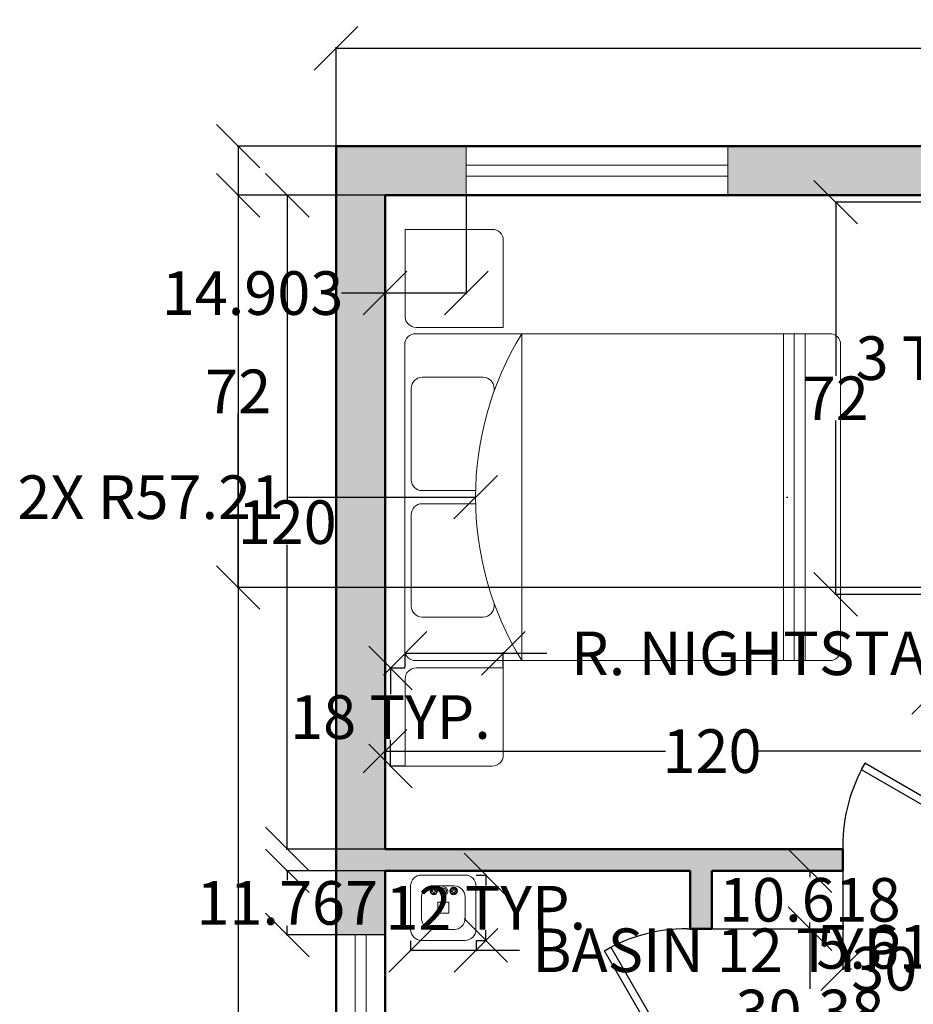
# Model space of a CAD drawing. Units: inches. Extents: x -87 to 308, y -349 to 42.
# Tile 2 of 6: x -45 to 119, y -139 to 42. Entities that reach past the tile are written whole.
import ezdxf

# ---------------------------------------------------------------- set-up
doc = ezdxf.new("R2010")
doc.units = ezdxf.units.IN
doc.header["$MEASUREMENT"] = 0
for name, color, linetype, lineweight in [('A-ANNO-DIMS', 2, 'Continuous', 18), ('A-DOOR', 3, 'Continuous', 25), ('A-FLOR-FIXT', 9, 'Continuous', 18), ('A-FURN', 8, 'Continuous', 18), ('A-GLAZ', 4, 'Continuous', 18), ('A-WALL', 7, 'Continuous', 50), ('A-WALL-PATT', 251, 'Continuous', 13)]:
    doc.layers.add(name, color=color, linetype=linetype, lineweight=lineweight)
doc.styles.get("Standard").update_dxf_attribs({"font": 'arial.ttf'})
doc.dimstyles.get("Standard").update_dxf_attribs({"dimtxt": 8, "dimasz": 8, "dimexe": 0.18, "dimexo": 0.0625, "dimgap": 0.09, "dimtad": 0, "dimtih": 1, "dimtoh": 1, "dimdec": 0, "dimzin": 0, "dimdsep": 46, "dimlunit": 4, "dimtxsty": 'Standard', "dimblk": 'OBLIQUE', "dimcen": 0.09, "dimadec": 0, "dimazin": 0, "dimtfac": 1, "dimtdec": 0, "dimtofl": 0, "dimtmove": 0, "dimatfit": 3, "dimldrblk": 'OBLIQUE', "dimfxl": 1, "dimtolj": 1, "dimtzin": 0, "dimarcsym": 0})

# ---------------------------------------------------------------- blocks, each defined once
blk = doc.blocks.new('*U6')
for p, q in [((-40, 0), (-40, 6)), ((0, 0), (0, 6))]:
    blk.add_line(p, q)
blk.add_lwpolyline([(0, 0), (-34.64, -20), (-35.52, -18.48), (-0.87, 1.52)], close=True)
blk.add_arc((0, 0), 40, 180, 210)
blk = doc.blocks.new('*U5')
for p, q in [((0, 0), (0, -6)), ((-40, 0), (-40, -6))]:
    blk.add_line(p, q)
blk.add_lwpolyline([(0, 0), (-34.64, 20), (-35.52, 18.48), (-0.88, -1.52)], close=True)
blk.add_arc((0, 0), 40, 150, 180)
blk = doc.blocks.new('Bed - Queen')
for p, q in [((2, 0), (58, 0)), ((10, -1.2), (26.8, -1.2)), ((33.2, -1.2), (50, -1.2)), ((0, -78), (0, -2)), ((8, -14.4), (8, -3.2)), ((28.8, -3.2), (28.8, -13.02)), ((31.2, -13.02), (31.2, -3.2)), ((52, -3.2), (52, -14.4)), ((60, -2), (60, -78)), ((10.58, -16.4), (10, -16.4)), ((50, -16.4), (49.42, -16.4)), ((60, -21.5), (0, -21.5)), ((0, -69.5), (60, -69.5)), ((0, -71.5), (60, -71.5)), ((0, -73.5), (60, -73.5)), ((58, -80), (2, -80))]:
    blk.add_line(p, q)
for centre, radius, start, end in [((58, -2), 2, 0, 90), ((2, -2), 2, 90, 180), ((10, -3.2), 2, 90, 180), ((26.8, -3.2), 2, 0, 90), ((33.2, -3.2), 2, 90, 180), ((50, -3.2), 2, 0, 90), ((30, -70.21), 57.21, 58.3725, 121.6275), ((10, -14.4), 2, 180, 270), ((50, -14.4), 2, 270, 0), ((2, -78), 2, 180, 270), ((58, -78), 2, 270, 0)]:
    blk.add_arc(centre, radius, start, end)
blk = doc.blocks.new('Faucet - Bathroom top')
for p, q in [((-4.107, 0.125), (-4.375, 0.125)), ((-3.75, 0.4788), (-3.75, 0.75)), ((-3.5, 0.482), (-3.5, 0.75)), ((-3.1461, 0.125), (-2.875, 0.125)), ((3.143, 0.125), (2.875, 0.125)), ((3.5, 0.4788), (3.5, 0.75)), ((3.75, 0.482), (3.75, 0.75)), ((4.1039, 0.125), (4.375, 0.125)), ((-4.1039, -0.125), (-4.375, -0.125)), ((-3.75, -0.4821), (-3.75, -0.75)), ((-3.5, -0.4789), (-3.5, -0.75)), ((-3.143, -0.125), (-2.875, -0.125)), ((-0.5, -0.8639), (-0.5, -4.5)), ((0.5, -4.5), (0.5, -0.8631)), ((3.1461, -0.125), (2.875, -0.125)), ((3.5, -0.4821), (3.5, -0.75)), ((3.75, -0.4789), (3.75, -0.75)), ((4.107, -0.125), (4.375, -0.125))]:
    blk.add_line(p, q)
for centre, radius in [((-3.625, 0), 1.375), ((-4.625, 0), 0.2795), ((-3.625, 0), 0.5), ((-3.625, 1), 0.2795), ((-2.625, 0), 0.2795), ((0, 0), 0.5), ((3.625, 0), 1.375), ((2.625, 0), 0.2795), ((3.625, 0), 0.5), ((3.625, 1), 0.2795), ((4.625, 0), 0.2795), ((-3.625, -1), 0.2795), ((3.625, -1), 0.2795)]:
    blk.add_circle(centre, radius)
for centre, radius, start, end in [((-3.625, 0), 1, 105.2407, 164.2093), ((-3.625, 0), 1, 16.44125, 74.07887), ((0, 0), 1.5, 289.6514, 250.3603), ((0, 0), 1, 300.3431, 239.7554), ((3.625, 0), 1, 106.12, 164.0884), ((3.625, 0), 1, 16.23422, 73.90469), ((-3.625, 0), 1, 196.2342, 253.9047), ((-3.625, 0), 1, 286.12, 344.0884), ((3.625, 0), 1, 196.4413, 254.0789), ((3.625, 0), 1, 285.2407, 344.2093), ((0, -4.5), 0.5, 180, 0)]:
    blk.add_arc(centre, radius, start, end)
blk = doc.blocks.new('WIN-48IN')
for p, q in [((0, 5.5), (48, 5.5)), ((0, 3.5), (48, 3.5))]:
    blk.add_line(p, q)
for points in [[(0, 0), (0, 9)], [(48, 9), (48, 0)]]:
    blk.add_lwpolyline(points)
blk = doc.blocks.new('WIN-24IN')
for p, q in [((0, 5.5), (24, 5.5)), ((0, 3.5), (24, 3.5))]:
    blk.add_line(p, q)
for points in [[(0, 0), (0, 9)], [(24, 9), (24, 0)]]:
    blk.add_lwpolyline(points)
blk = doc.blocks.new('LAVATORY-12IN')
for p, q in [((2, 12), (10, 12)), ((0, 2), (0, 10)), ((4, 10), (8, 10)), ((12, 10), (12, 2)), ((2, 4), (2, 8)), ((10, 8), (10, 4)), ((5, 7), (7, 7)), ((5, 5), (5, 7)), ((7, 7), (7, 5)), ((7, 5), (5, 5)), ((8, 2), (4, 2)), ((10, 0), (2, 0))]:
    blk.add_line(p, q)
for centre, start, end in [((2, 10), 90, 180), ((10, 10), 0, 90), ((4, 8), 90, 180), ((8, 8), 0, 90), ((4, 4), 180, 270), ((8, 4), 270, 0), ((2, 2), 180, 270), ((10, 2), 270, 0)]:
    blk.add_arc(centre, 2, start, end)
blk = doc.blocks.new('NIGHTSTAND-18IN-L')
blk.add_lwpolyline([(2, 0), (18, 0), (18, 16, 0.414214), (16, 18), (0, 18), (0, 2, 0.414214)], format="xyb", close=True)
blk = doc.blocks.new('NIGHTSTAND-18IN-R')
blk.add_lwpolyline([(0, 0), (16, 0, 0.414214), (18, 2), (18, 18), (2, 18, 0.414214), (0, 16)], format="xyb", close=True)
blk = doc.blocks.new('_Oblique')
at = {"color": 0, "linetype": 'ByBlock', "lineweight": -2}
blk.add_line((-0.5, -0.5), (0.5, 0.5), dxfattribs=at)
blk = doc.blocks.new('*D32')
at = {"layer": 'A-ANNO-DIMS', "color": 0, "lineweight": -2, "transparency": 16777216}
for p, q in [((147.96, -20.57), (139.96, -20.57)), ((147.96, -21.27), (147.96, -20.39)), ((151.23, -20.57), (147.96, -20.57)), ((151.23, -21.27), (151.23, -20.39))]:
    blk.add_line(p, q, dxfattribs=at)
at = {"layer": 'Defpoints', "color": 0, "transparency": 16777216}
for p in [(147.96, -20.57), (147.96, -21.33), (151.23, -21.33)]:
    blk.add_point(p, dxfattribs=at)
at = {"layer": 'A-ANNO-DIMS', "color": 0, "lineweight": -2, "transparency": 16777216, "xscale": 8, "yscale": 8, "zscale": 8, "rotation": 180}
blk.add_blockref('_Oblique', (147.96, -20.57), dxfattribs=at)
at = {"layer": 'A-ANNO-DIMS', "color": 0, "lineweight": -2, "transparency": 16777216, "xscale": 8, "yscale": 8, "zscale": 8}
blk.add_blockref('_Oblique', (151.23, -20.57), dxfattribs=at)
at = {"layer": 'A-ANNO-DIMS', "color": 0, "transparency": 16777216, "insert": (123.51, -20.57), "char_height": 8, "attachment_point": 5}
blk.add_mtext('\\A1;3 TYP.', dxfattribs=at)
blk = doc.blocks.new('*D33')
at = {"layer": 'A-ANNO-DIMS', "color": 0, "lineweight": -2, "transparency": 16777216}
for p, q in [((26.45, -127.5), (26.45, -129.42)), ((38.45, -127.5), (38.45, -129.42)), ((26.45, -129.24), (38.45, -129.24)), ((38.45, -129.24), (46.45, -129.24))]:
    blk.add_line(p, q, dxfattribs=at)
at = {"layer": 'Defpoints', "color": 0, "transparency": 16777216}
for p in [(26.45, -127.44), (38.45, -127.44), (38.45, -129.24)]:
    blk.add_point(p, dxfattribs=at)
at = {"layer": 'A-ANNO-DIMS', "color": 0, "lineweight": -2, "transparency": 16777216, "xscale": 8, "yscale": 8, "zscale": 8, "rotation": 180}
blk.add_blockref('_Oblique', (26.45, -129.24), dxfattribs=at)
at = {"layer": 'A-ANNO-DIMS', "color": 0, "lineweight": -2, "transparency": 16777216, "xscale": 8, "yscale": 8, "zscale": 8}
blk.add_blockref('_Oblique', (38.45, -129.24), dxfattribs=at)
at = {"layer": 'A-ANNO-DIMS', "color": 0, "transparency": 16777216, "insert": (84.15, -129.24), "char_height": 8, "attachment_point": 5}
blk.add_mtext('\\A1;BASIN 12 TYP.', dxfattribs=at)
blk = doc.blocks.new('*D34')
at = {"layer": 'A-ANNO-DIMS', "color": 0, "lineweight": -2, "transparency": 16777216}
for p, q in [((38.51, -115.44), (40.43, -115.44)), ((40.25, -115.44), (40.25, -117.33)), ((40.25, -127.44), (40.25, -125.54)), ((38.51, -127.44), (40.43, -127.44))]:
    blk.add_line(p, q, dxfattribs=at)
at = {"layer": 'Defpoints', "color": 0, "transparency": 16777216}
for p in [(38.45, -115.44), (40.25, -115.44), (38.45, -127.44)]:
    blk.add_point(p, dxfattribs=at)
at = {"layer": 'A-ANNO-DIMS', "color": 0, "lineweight": -2, "transparency": 16777216, "xscale": 8, "yscale": 8, "zscale": 8}
for p, rotation in [((40.25, -115.44), 90), ((40.25, -127.44), 270)]:
    blk.add_blockref('_Oblique', p, dxfattribs=dict(at, rotation=rotation))
at = {"layer": 'A-ANNO-DIMS', "color": 0, "transparency": 16777216, "insert": (40.25, -121.44), "char_height": 8, "attachment_point": 5}
blk.add_mtext('\\A1;12 TYP.', dxfattribs=at)
blk = doc.blocks.new('*D37')
at = {"layer": 'A-ANNO-DIMS', "color": 0, "lineweight": -2, "transparency": 16777216}
for p, q in [((25.45, -77.37), (25.45, -74.56)), ((25.45, -74.74), (43.45, -74.74)), ((43.45, -77.37), (43.45, -74.56)), ((43.45, -74.74), (51.45, -74.74))]:
    blk.add_line(p, q, dxfattribs=at)
at = {"layer": 'Defpoints', "color": 0, "transparency": 16777216}
for p in [(43.45, -74.74), (25.45, -77.44), (43.45, -77.44)]:
    blk.add_point(p, dxfattribs=at)
at = {"layer": 'A-ANNO-DIMS', "color": 0, "lineweight": -2, "transparency": 16777216, "xscale": 8, "yscale": 8, "zscale": 8, "rotation": 180}
blk.add_blockref('_Oblique', (25.45, -74.74), dxfattribs=at)
at = {"layer": 'A-ANNO-DIMS', "color": 0, "lineweight": -2, "transparency": 16777216, "xscale": 8, "yscale": 8, "zscale": 8}
blk.add_blockref('_Oblique', (43.45, -74.74), dxfattribs=at)
at = {"layer": 'A-ANNO-DIMS', "color": 0, "transparency": 16777216, "insert": (115.81, -74.74), "char_height": 8, "attachment_point": 5}
blk.add_mtext('\\A1;R. NIGHTSTAND 18 TYP.', dxfattribs=at)
blk = doc.blocks.new('*D38')
at = {"layer": 'A-ANNO-DIMS', "color": 0, "lineweight": -2, "transparency": 16777216}
for p, q in [((25.38, -77.44), (22.57, -77.44)), ((22.75, -77.44), (22.75, -82.26)), ((22.75, -95.44), (22.75, -90.61)), ((25.38, -95.44), (22.57, -95.44))]:
    blk.add_line(p, q, dxfattribs=at)
at = {"layer": 'Defpoints', "color": 0, "transparency": 16777216}
for p in [(22.75, -77.44), (25.45, -77.44), (25.45, -95.44)]:
    blk.add_point(p, dxfattribs=at)
at = {"layer": 'A-ANNO-DIMS', "color": 0, "lineweight": -2, "transparency": 16777216, "xscale": 8, "yscale": 8, "zscale": 8}
for p, rotation in [((22.75, -77.44), 90), ((22.75, -95.44), 270)]:
    blk.add_blockref('_Oblique', p, dxfattribs=dict(at, rotation=rotation))
at = {"layer": 'A-ANNO-DIMS', "color": 0, "transparency": 16777216, "insert": (22.75, -86.44), "char_height": 8, "attachment_point": 5}
blk.add_mtext('\\A1;18 TYP.', dxfattribs=at)
blk = doc.blocks.new('*D47')
at = {"layer": 'A-ANNO-DIMS', "color": 0, "lineweight": -2, "transparency": 16777216}
for p, q in [((12.76, 18.39), (12.76, 36.48)), ((12.76, 36.3), (120.78, 36.3)), ((246.76, 36.3), (138.74, 36.3)), ((246.76, 18.39), (246.76, 36.48))]:
    blk.add_line(p, q, dxfattribs=at)
at = {"layer": 'Defpoints', "color": 0, "transparency": 16777216}
for p in [(246.76, 36.3), (12.76, 18.33), (246.76, 18.33)]:
    blk.add_point(p, dxfattribs=at)
at = {"layer": 'A-ANNO-DIMS', "color": 0, "lineweight": -2, "transparency": 16777216, "xscale": 8, "yscale": 8, "zscale": 8, "rotation": 180}
blk.add_blockref('_Oblique', (12.76, 36.3), dxfattribs=at)
at = {"layer": 'A-ANNO-DIMS', "color": 0, "lineweight": -2, "transparency": 16777216, "xscale": 8, "yscale": 8, "zscale": 8}
blk.add_blockref('_Oblique', (246.76, 36.3), dxfattribs=at)
at = {"layer": 'A-ANNO-DIMS', "color": 0, "transparency": 16777216, "insert": (129.76, 36.3), "char_height": 8, "attachment_point": 5}
blk.add_mtext('\\A1;234', dxfattribs=at)
blk = doc.blocks.new('*D48')
at = {"layer": 'A-ANNO-DIMS', "color": 0, "lineweight": -2, "transparency": 16777216}
for p, q in [((12.7, 18.33), (-5.38, 18.33)), ((-5.2, 18.33), (-5.2, -148.49)), ((-5.2, -323.67), (-5.2, -156.85)), ((12.7, -323.67), (-5.38, -323.67))]:
    blk.add_line(p, q, dxfattribs=at)
at = {"layer": 'Defpoints', "color": 0, "transparency": 16777216}
for p in [(-5.2, 18.33), (12.76, 18.33), (12.76, -323.67)]:
    blk.add_point(p, dxfattribs=at)
at = {"layer": 'A-ANNO-DIMS', "color": 0, "lineweight": -2, "transparency": 16777216, "xscale": 8, "yscale": 8, "zscale": 8}
for p, rotation in [((-5.2, 18.33), 90), ((-5.2, -323.67), 270)]:
    blk.add_blockref('_Oblique', p, dxfattribs=dict(at, rotation=rotation))
at = {"layer": 'A-ANNO-DIMS', "color": 0, "transparency": 16777216, "insert": (-5.2, -152.67), "char_height": 8, "attachment_point": 5}
blk.add_mtext('\\A1;342', dxfattribs=at)
blk = doc.blocks.new('*D49')
at = {"layer": 'A-ANNO-DIMS', "color": 0, "lineweight": -2, "transparency": 16777216}
for p, q in [((21.76, 9.27), (21.76, -8.81)), ((36.67, 9.27), (36.67, -8.81)), ((21.76, -8.63), (13.76, -8.63)), ((36.67, -8.63), (21.76, -8.63))]:
    blk.add_line(p, q, dxfattribs=at)
at = {"layer": 'Defpoints', "color": 0, "transparency": 16777216}
for p in [(21.76, 9.33), (36.67, 9.33), (21.76, -8.63)]:
    blk.add_point(p, dxfattribs=at)
at = {"layer": 'A-ANNO-DIMS', "color": 0, "lineweight": -2, "transparency": 16777216, "xscale": 8, "yscale": 8, "zscale": 8}
for p, rotation in [((21.76, -8.63), 179.9999999999999), ((36.67, -8.63), 359.9999999999999)]:
    blk.add_blockref('_Oblique', p, dxfattribs=dict(at, rotation=rotation))
at = {"layer": 'A-ANNO-DIMS', "color": 0, "transparency": 16777216, "insert": (-2.56, -8.63), "char_height": 8, "attachment_point": 5}
blk.add_mtext('\\A1;14.903', dxfattribs=at)
blk = doc.blocks.new('*D55')
at = {"layer": 'A-ANNO-DIMS', "color": 0, "lineweight": -2, "transparency": 16777216}
for p, q in [((21.7, -114.67), (3.62, -114.67)), ((3.8, -114.67), (3.8, -116.38)), ((21.7, -126.44), (3.62, -126.44)), ((3.8, -126.44), (3.8, -124.73))]:
    blk.add_line(p, q, dxfattribs=at)
at = {"layer": 'Defpoints', "color": 0, "transparency": 16777216}
for p in [(3.8, -114.67), (21.76, -114.67), (21.76, -126.44)]:
    blk.add_point(p, dxfattribs=at)
at = {"layer": 'A-ANNO-DIMS', "color": 0, "lineweight": -2, "transparency": 16777216, "xscale": 8, "yscale": 8, "zscale": 8}
for p, rotation in [((3.8, -114.67), 90), ((3.8, -126.44), 270)]:
    blk.add_blockref('_Oblique', p, dxfattribs=dict(at, rotation=rotation))
at = {"layer": 'A-ANNO-DIMS', "color": 0, "transparency": 16777216, "insert": (3.8, -120.55), "char_height": 8, "attachment_point": 5}
blk.add_mtext('\\A1;11.767', dxfattribs=at)
blk = doc.blocks.new('*D58')
at = {"layer": 'A-ANNO-DIMS', "color": 0, "lineweight": -2, "transparency": 16777216}
for p, q in [((21.76, -110.61), (21.76, -92.52)), ((21.76, -92.7), (73.23, -92.7)), ((141.76, -92.7), (90.3, -92.7)), ((141.76, -110.61), (141.76, -92.52))]:
    blk.add_line(p, q, dxfattribs=at)
at = {"layer": 'Defpoints', "color": 0, "transparency": 16777216}
for p in [(141.76, -92.7), (21.76, -110.67), (141.76, -110.67)]:
    blk.add_point(p, dxfattribs=at)
at = {"layer": 'A-ANNO-DIMS', "color": 0, "lineweight": -2, "transparency": 16777216, "xscale": 8, "yscale": 8, "zscale": 8, "rotation": 180}
blk.add_blockref('_Oblique', (21.76, -92.7), dxfattribs=at)
at = {"layer": 'A-ANNO-DIMS', "color": 0, "lineweight": -2, "transparency": 16777216, "xscale": 8, "yscale": 8, "zscale": 8}
blk.add_blockref('_Oblique', (141.76, -92.7), dxfattribs=at)
at = {"layer": 'A-ANNO-DIMS', "color": 0, "transparency": 16777216, "insert": (81.76, -92.7), "char_height": 8, "attachment_point": 5}
blk.add_mtext('\\A1;120', dxfattribs=at)
blk = doc.blocks.new('*D59')
at = {"layer": 'A-ANNO-DIMS', "color": 0, "lineweight": -2, "transparency": 16777216}
for p, q in [((21.7, 9.33), (3.62, 9.33)), ((3.8, 9.33), (3.8, -46.49)), ((3.8, -110.67), (3.8, -54.84)), ((21.7, -110.67), (3.62, -110.67))]:
    blk.add_line(p, q, dxfattribs=at)
at = {"layer": 'Defpoints', "color": 0, "transparency": 16777216}
for p in [(3.8, 9.33), (21.76, 9.33), (21.76, -110.67)]:
    blk.add_point(p, dxfattribs=at)
at = {"layer": 'A-ANNO-DIMS', "color": 0, "lineweight": -2, "transparency": 16777216, "xscale": 8, "yscale": 8, "zscale": 8}
for p, rotation in [((3.8, 9.33), 90), ((3.8, -110.67), 270)]:
    blk.add_blockref('_Oblique', p, dxfattribs=dict(at, rotation=rotation))
at = {"layer": 'A-ANNO-DIMS', "color": 0, "transparency": 16777216, "insert": (3.8, -50.67), "char_height": 8, "attachment_point": 5}
blk.add_mtext('\\A1;120', dxfattribs=at)
blk = doc.blocks.new('*D60')
at = {"layer": 'A-ANNO-DIMS', "color": 0, "lineweight": -2, "transparency": 16777216}
for p, q in [((145.7, 9.33), (-5.38, 9.33)), ((-5.2, 9.33), (-5.2, -22.56)), ((-5.2, -62.67), (-5.2, -30.77)), ((145.7, -62.67), (-5.38, -62.67))]:
    blk.add_line(p, q, dxfattribs=at)
at = {"layer": 'Defpoints', "color": 0, "transparency": 16777216}
for p in [(-5.2, 9.33), (145.76, 9.33), (145.76, -62.67)]:
    blk.add_point(p, dxfattribs=at)
at = {"layer": 'A-ANNO-DIMS', "color": 0, "lineweight": -2, "transparency": 16777216, "xscale": 8, "yscale": 8, "zscale": 8}
for p, rotation in [((-5.2, 9.33), 90), ((-5.2, -62.67), 270)]:
    blk.add_blockref('_Oblique', p, dxfattribs=dict(at, rotation=rotation))
at = {"layer": 'A-ANNO-DIMS', "color": 0, "transparency": 16777216, "insert": (-5.2, -26.67), "char_height": 8, "attachment_point": 5}
blk.add_mtext('\\A1;72', dxfattribs=at)
blk = doc.blocks.new('*D66')
at = {"layer": 'A-ANNO-DIMS', "color": 0, "lineweight": -2, "transparency": 16777216}
for p, q in [((105.76, -114.73), (105.76, -132.81)), ((136.15, -114.73), (136.15, -132.81)), ((105.76, -132.63), (107.36, -132.63)), ((136.15, -132.63), (134.55, -132.63))]:
    blk.add_line(p, q, dxfattribs=at)
at = {"layer": 'Defpoints', "color": 0, "transparency": 16777216}
for p in [(105.76, -114.67), (136.15, -114.67), (105.76, -132.63)]:
    blk.add_point(p, dxfattribs=at)
at = {"layer": 'A-ANNO-DIMS', "color": 0, "lineweight": -2, "transparency": 16777216, "xscale": 8, "yscale": 8, "zscale": 8, "rotation": 180}
blk.add_blockref('_Oblique', (105.76, -132.63), dxfattribs=at)
at = {"layer": 'A-ANNO-DIMS', "color": 0, "lineweight": -2, "transparency": 16777216, "xscale": 8, "yscale": 8, "zscale": 8}
blk.add_blockref('_Oblique', (136.15, -132.63), dxfattribs=at)
at = {"layer": 'A-ANNO-DIMS', "color": 0, "transparency": 16777216, "insert": (120.95, -132.63), "char_height": 8, "attachment_point": 5}
blk.add_mtext('\\A1;30.38', dxfattribs=at)
blk = doc.blocks.new('*D67')
at = {"layer": 'A-ANNO-DIMS', "color": 0, "lineweight": -2, "transparency": 16777216}
for p, q in [((136.15, -110.73), (136.15, -128.81)), ((141.76, -110.73), (141.76, -128.81)), ((136.15, -128.63), (128.15, -128.63)), ((141.76, -128.63), (136.15, -128.63))]:
    blk.add_line(p, q, dxfattribs=at)
at = {"layer": 'Defpoints', "color": 0, "transparency": 16777216}
for p in [(136.15, -110.67), (141.76, -110.67), (136.15, -128.63)]:
    blk.add_point(p, dxfattribs=at)
at = {"layer": 'A-ANNO-DIMS', "color": 0, "lineweight": -2, "transparency": 16777216, "xscale": 8, "yscale": 8, "zscale": 8, "rotation": 180}
blk.add_blockref('_Oblique', (136.15, -128.63), dxfattribs=at)
at = {"layer": 'A-ANNO-DIMS', "color": 0, "lineweight": -2, "transparency": 16777216, "xscale": 8, "yscale": 8, "zscale": 8}
blk.add_blockref('_Oblique', (141.76, -128.63), dxfattribs=at)
at = {"layer": 'A-ANNO-DIMS', "color": 0, "transparency": 16777216, "insert": (114.55, -128.63), "char_height": 8, "attachment_point": 5}
blk.add_mtext('\\A1;5.618', dxfattribs=at)
blk = doc.blocks.new('*D70')
at = {"layer": 'A-ANNO-DIMS', "color": 0, "lineweight": -2, "transparency": 16777216}
for p, q in [((81.83, -125.29), (99.91, -125.29)), ((99.73, -125.29), (99.73, -136.3)), ((99.73, -155.67), (99.73, -144.65)), ((81.83, -155.67), (99.91, -155.67))]:
    blk.add_line(p, q, dxfattribs=at)
at = {"layer": 'Defpoints', "color": 0, "transparency": 16777216}
for p in [(81.76, -125.29), (81.76, -155.67), (99.73, -155.67)]:
    blk.add_point(p, dxfattribs=at)
at = {"layer": 'A-ANNO-DIMS', "color": 0, "lineweight": -2, "transparency": 16777216, "xscale": 8, "yscale": 8, "zscale": 8}
for p, rotation in [((99.73, -125.29), 90), ((99.73, -155.67), 270)]:
    blk.add_blockref('_Oblique', p, dxfattribs=dict(at, rotation=rotation))
at = {"layer": 'A-ANNO-DIMS', "color": 0, "transparency": 16777216, "insert": (99.73, -140.48), "char_height": 8, "attachment_point": 5}
blk.add_mtext('\\A1;30.38', dxfattribs=at)
blk = doc.blocks.new('*D71')
at = {"layer": 'A-ANNO-DIMS', "color": 0, "lineweight": -2, "transparency": 16777216}
for p, q in [((81.83, -114.67), (99.91, -114.67)), ((99.73, -114.67), (99.73, -115.8)), ((99.73, -125.29), (99.73, -124.15)), ((81.83, -125.29), (99.91, -125.29))]:
    blk.add_line(p, q, dxfattribs=at)
at = {"layer": 'Defpoints', "color": 0, "transparency": 16777216}
for p in [(81.76, -114.67), (81.76, -125.29), (99.73, -125.29)]:
    blk.add_point(p, dxfattribs=at)
at = {"layer": 'A-ANNO-DIMS', "color": 0, "lineweight": -2, "transparency": 16777216, "xscale": 8, "yscale": 8, "zscale": 8}
for p, rotation in [((99.73, -114.67), 90), ((99.73, -125.29), 270)]:
    blk.add_blockref('_Oblique', p, dxfattribs=dict(at, rotation=rotation))
at = {"layer": 'A-ANNO-DIMS', "color": 0, "transparency": 16777216, "insert": (99.73, -119.98), "char_height": 8, "attachment_point": 5}
blk.add_mtext('\\A1;10.618', dxfattribs=at)
blk = doc.blocks.new('*D81')
at = {"layer": 'A-ANNO-DIMS', "color": 0, "lineweight": -2, "transparency": 16777216}
for p, q in [((122.45, -64), (122.45, -82.08)), ((140.45, -64), (140.45, -82.08)), ((122.45, -81.9), (125.99, -81.9)), ((140.45, -81.9), (136.9, -81.9))]:
    blk.add_line(p, q, dxfattribs=at)
at = {"layer": 'Defpoints', "color": 0, "transparency": 16777216}
for p in [(122.45, -63.94), (140.45, -63.94), (122.45, -81.9)]:
    blk.add_point(p, dxfattribs=at)
at = {"layer": 'A-ANNO-DIMS', "color": 0, "lineweight": -2, "transparency": 16777216, "xscale": 8, "yscale": 8, "zscale": 8, "rotation": 180}
blk.add_blockref('_Oblique', (122.45, -81.9), dxfattribs=at)
at = {"layer": 'A-ANNO-DIMS', "color": 0, "lineweight": -2, "transparency": 16777216, "xscale": 8, "yscale": 8, "zscale": 8}
blk.add_blockref('_Oblique', (140.45, -81.9), dxfattribs=at)
at = {"layer": 'A-ANNO-DIMS', "color": 0, "transparency": 16777216, "insert": (131.45, -81.9), "char_height": 8, "attachment_point": 5}
blk.add_mtext('\\A1;18', dxfattribs=at)
blk = doc.blocks.new('*D82')
at = {"layer": 'A-ANNO-DIMS', "color": 0, "lineweight": -2, "transparency": 16777216}
for p, q in [((122.38, 8.06), (104.3, 8.06)), ((104.48, 8.06), (104.48, -23.83)), ((104.48, -63.94), (104.48, -32.04)), ((122.38, -63.94), (104.3, -63.94))]:
    blk.add_line(p, q, dxfattribs=at)
at = {"layer": 'Defpoints', "color": 0, "transparency": 16777216}
for p in [(104.48, 8.06), (122.45, 8.06), (122.45, -63.94)]:
    blk.add_point(p, dxfattribs=at)
at = {"layer": 'A-ANNO-DIMS', "color": 0, "lineweight": -2, "transparency": 16777216, "xscale": 8, "yscale": 8, "zscale": 8}
for p, rotation in [((104.48, 8.06), 90), ((104.48, -63.94), 270)]:
    blk.add_blockref('_Oblique', p, dxfattribs=dict(at, rotation=rotation))
at = {"layer": 'A-ANNO-DIMS', "color": 0, "transparency": 16777216, "insert": (104.48, -27.94), "char_height": 8, "attachment_point": 5}
blk.add_mtext('\\A1;72', dxfattribs=at)
blk = doc.blocks.new('*D95')
at = {"layer": 'A-ANNO-DIMS', "color": 0, "lineweight": -2, "transparency": 16777216}
for p, q in [((4.04, -46.09), (38.37, -46.09)), ((95.49, -46.09), (95.67, -46.09)), ((95.58, -46.18), (95.58, -46))]:
    blk.add_line(p, q, dxfattribs=at)
at = {"layer": 'Defpoints', "color": 0, "transparency": 16777216}
for p in [(38.37, -46.09), (95.58, -46.09)]:
    blk.add_point(p, dxfattribs=at)
at = {"layer": 'A-ANNO-DIMS', "color": 0, "lineweight": -2, "transparency": 16777216, "xscale": 8, "yscale": 8, "zscale": 8, "rotation": 359.9998577843114}
blk.add_blockref('_Oblique', (38.37, -46.09), dxfattribs=at)
at = {"layer": 'A-ANNO-DIMS', "color": 0, "transparency": 16777216, "insert": (-21.26, -46.09), "char_height": 8, "attachment_point": 5}
blk.add_mtext('\\A1;2X R57.21', dxfattribs=at)

msp = doc.modelspace()

# ---------------------------------------------------------------- hatches: boundary and pattern name
at = {"layer": 'A-WALL-PATT'}
h = msp.add_hatch(color=256, dxfattribs=at)
h.dxf.hatch_style = 1
h.paths.add_polyline_path([(36.6671, 18.332), (12.7637, 18.332), (12.7637, -126.4351), (21.7637, -126.4351), (21.7637, -114.668), (77.7637, -114.668), (77.7637, -125.2857), (81.7637, -125.2857), (81.7637, -114.668), (105.7637, -114.668), (105.7637, -110.668), (21.7637, -110.668), (21.7637, 9.332), (36.6671, 9.332)])
h = msp.add_hatch(color=256, dxfattribs=at)
h.dxf.hatch_style = 1
h.paths.add_polyline_path([(184.748, 18.332), (84.6671, 18.332), (84.6671, 9.332), (141.7637, 9.332), (141.7637, -110.668), (136.146, -110.668), (136.146, -114.668), (145.7637, -114.668), (145.7637, -66.668), (151.7637, -66.668), (151.7637, -62.668), (145.7637, -62.668), (145.7637, 9.332), (184.748, 9.332)])

# ---------------------------------------------------------------- linework, layer by layer
at = {"layer": 'A-WALL'}
for p, q in [((21.7637, 9.332), (141.7637, 9.332)), ((21.7637, -110.668), (21.7637, 9.332)), ((21.7637, -110.668), (105.7637, -110.668)), ((105.7637, -110.668), (105.7637, -114.668)), ((21.7637, -114.668), (77.7637, -114.668)), ((21.7637, -166.668), (21.7637, -114.668)), ((77.7637, -125.2857), (77.7637, -114.668)), ((81.7637, -114.668), (105.7637, -114.668)), ((81.7637, -125.2857), (81.7637, -114.668)), ((77.7637, -125.2857), (81.7637, -125.2857))]:
    msp.add_line(p, q, dxfattribs=at)
msp.add_lwpolyline([(142.7127, -323.668), (12.7637, -323.668), (12.7637, 18.332), (246.7637, 18.332), (246.7637, -323.668), (172.7127, -323.668)], dxfattribs=at)

# ---------------------------------------------------------------- block references
at = {"layer": 'A-DOOR', "xscale": 0.7595575434647344, "yscale": 0.7595575434647344, "zscale": 0.7595575434647344}
msp.add_blockref('*U5', (136.146, -110.1107), dxfattribs=at)
at = {"layer": 'A-DOOR', "xscale": 0.7595575434647344, "yscale": 0.7595575434647344, "zscale": 0.7595575434647344, "rotation": 270}
msp.add_blockref('*U6', (77.2063, -155.668), dxfattribs=at)
at = {"layer": 'A-FLOR-FIXT'}
msp.add_blockref('LAVATORY-12IN', (26.4469, -127.435), dxfattribs=at)
at = {"layer": 'A-FLOR-FIXT', "xscale": 0.5034362513714087, "yscale": 0.5034362513714087, "zscale": 0.5034362513714087}
msp.add_blockref('Faucet - Bathroom top', (32.5346, -118.3822), dxfattribs=at)
at = {"layer": 'A-FURN'}
for name, p in [('NIGHTSTAND-18IN-L', (25.447, -14.935)), ('NIGHTSTAND-18IN-R', (25.447, -95.435))]:
    msp.add_blockref(name, p, dxfattribs=at)
at = {"layer": 'A-FURN', "rotation": 90}
msp.add_blockref('Bed - Queen', (25.3666, -76.0911), dxfattribs=at)
at = {"layer": 'A-GLAZ'}
msp.add_blockref('WIN-48IN', (36.667, 9.332), dxfattribs=at)
at = {"layer": 'A-GLAZ', "rotation": 270}
msp.add_blockref('WIN-24IN', (12.7637, -126.4351), dxfattribs=at)

# ---------------------------------------------------------------- dimensions: what is measured, and where the dimension line sits
at = {"layer": 'A-ANNO-DIMS'}
for base, p1, p2, picture, middle in [((246.7637, 36.2965), (12.7637, 18.332), (246.7637, 18.332), '*D47', (129.7637, 36.2965)), ((141.7637, -92.7035), (21.7637, -110.668), (141.7637, -110.668), '*D58', (81.7637, -92.7035))]:
    dim = msp.add_linear_dim(base=base, p1=p1, p2=p2, dimstyle='Standard', override={"dimdec": 0, "dimlfac": 1, "dimrnd": 0, "dimzin": 0, "dimdsep": 46, "dimlunit": 2}, dxfattribs=at)
    dim.commit()
    dim.dimension.update_dxf_attribs({"geometry": picture, "text_midpoint": middle})
for base, p1, p2, angle, override, picture, middle in [((-5.2008, 18.332), (12.7637, -323.668), (12.7637, 18.332), 90, {"dimdec": 0, "dimlfac": 1, "dimrnd": 0, "dimzin": 0, "dimdsep": 46, "dimlunit": 2}, '*D48', (-5.2008, -152.668)), ((-5.2008, 9.332), (145.7637, -62.668), (145.7637, 9.332), 90, {"dimdec": 0, "dimlfac": 1, "dimrnd": 0, "dimzin": 0, "dimdsep": 46, "dimlunit": 2}, '*D60', (-5.2008, -26.668)), ((3.7992, 9.332), (21.7637, -110.668), (21.7637, 9.332), 90, {"dimdec": 0, "dimlfac": 1, "dimrnd": 0, "dimzin": 0, "dimdsep": 46, "dimlunit": 2}, '*D59', (3.7992, -50.668)), ((104.482, 8.0649), (122.4465, -63.9351), (122.4465, 8.0649), 90, {"dimdec": 0, "dimlfac": 1, "dimrnd": 0, "dimzin": 0, "dimdsep": 46, "dimlunit": 2}, '*D82', (104.482, -27.9351)), ((21.7637, -8.6325), (36.6671, 9.332), (21.7637, 9.332), 180, {"dimdec": 3, "dimlfac": 1, "dimrnd": 0, "dimzin": 0, "dimdsep": 46, "dimlunit": 2}, '*D49', (-2.5555, -8.6325)), ((122.4465, -81.8996), (140.4465, -63.9351), (122.4465, -63.9351), 180, {"dimdec": 0, "dimlfac": 1, "dimrnd": 0, "dimzin": 0, "dimdsep": 46, "dimlunit": 2}, '*D81', (131.4465, -81.8996)), ((3.7992, -114.668), (21.7637, -126.4351), (21.7637, -114.668), 90, {"dimdec": 3, "dimlfac": 1, "dimrnd": 0, "dimzin": 0, "dimdsep": 46, "dimlunit": 2}, '*D55', (3.7992, -120.5516)), ((99.7282, -125.2857), (81.7637, -114.668), (81.7637, -125.2857), 270, {"dimdec": 3, "dimlfac": 1, "dimrnd": 0, "dimzin": 0, "dimdsep": 46, "dimlunit": 2}, '*D71', (99.7282, -119.9769)), ((136.146, -128.6325), (141.7637, -110.668), (136.146, -110.668), 180, {"dimdec": 3, "dimlfac": 1, "dimrnd": 0, "dimzin": 0, "dimdsep": 46, "dimlunit": 2}, '*D67', (114.5498, -128.6325)), ((105.7637, -132.6325), (136.146, -114.668), (105.7637, -114.668), 180, {"dimdec": 2, "dimlfac": 1, "dimrnd": 0, "dimzin": 0, "dimdsep": 46, "dimlunit": 2}, '*D66', (120.9548, -132.6325)), ((99.7282, -155.668), (81.7637, -125.2857), (81.7637, -155.668), 270, {"dimdec": 2, "dimlfac": 1, "dimrnd": 0, "dimzin": 0, "dimdsep": 46, "dimlunit": 2}, '*D70', (99.7282, -140.4769))]:
    dim = msp.add_linear_dim(base=base, p1=p1, p2=p2, angle=angle, dimstyle='Standard', override=override, dxfattribs=at)
    dim.commit()
    dim.dimension.update_dxf_attribs({"geometry": picture, "text_midpoint": middle})
for base, p1, p2, angle, picture, middle in [((147.9555, -20.5747), (151.2279, -21.3298), (147.9555, -21.3298), 180, '*D32', (123.5054, -20.5747)), ((22.7465, -77.4351), (25.4465, -95.4351), (25.4465, -77.4351), 90, '*D38', (22.7465, -86.4351)), ((40.2465, -115.4351), (38.4465, -127.4351), (38.4465, -115.4351), 90, '*D34', (40.2465, -121.4351))]:
    dim = msp.add_linear_dim(base=base, p1=p1, p2=p2, angle=angle, text='<> TYP.', dimstyle='Standard', override={"dimdec": 0, "dimlfac": 1, "dimrnd": 0, "dimzin": 0, "dimdsep": 46, "dimlunit": 2}, dxfattribs=at)
    dim.commit()
    dim.dimension.update_dxf_attribs({"geometry": picture, "text_midpoint": middle})
dim = msp.add_radius_dim(center=(95.5785, -46.0911), mpoint=(38.3697, -46.091), text='2X <>', dimstyle='Standard', override={"dimdec": 2, "dimlfac": 1, "dimrnd": 0, "dimzin": 0, "dimdsep": 46, "dimlunit": 2}, dxfattribs=at)
dim.commit()
dim.dimension.update_dxf_attribs({"geometry": '*D95', "text_midpoint": (4.0443, -46.0909), "dimtype": 164})
for base, p1, p2, text, picture, middle in [((43.4465, -74.7351), (25.4465, -77.4351), (43.4465, -77.4351), 'R. NIGHTSTAND <> TYP.', '*D37', (115.8148, -74.7351)), ((38.4465, -129.2351), (26.4465, -127.4351), (38.4465, -127.4351), 'BASIN <> TYP.', '*D33', (84.1518, -129.2351))]:
    dim = msp.add_linear_dim(base=base, p1=p1, p2=p2, text=text, dimstyle='Standard', override={"dimdec": 0, "dimlfac": 1, "dimrnd": 0, "dimzin": 0, "dimdsep": 46, "dimlunit": 2}, dxfattribs=at)
    dim.commit()
    dim.dimension.update_dxf_attribs({"geometry": picture, "text_midpoint": middle})

doc.saveas('drawing.dxf')
